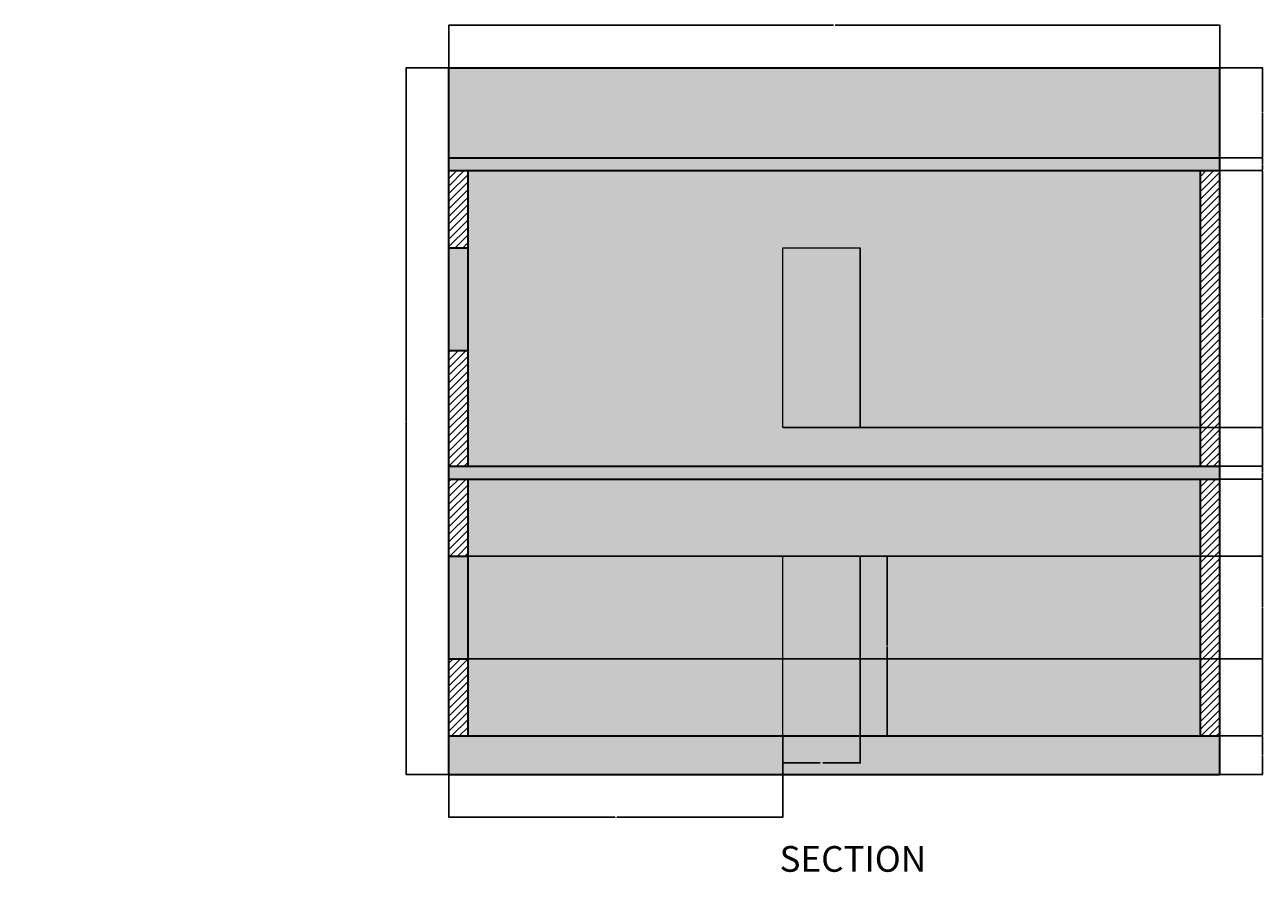
# Model space of a CAD drawing. Units: inches. Extents: x -43 to 1296, y -568 to 542.
# Tile 14 of 14: x 626 to 1204, y 83 to 479. Entities that reach past the tile are written whole.
import ezdxf

# ---------------------------------------------------------------- set-up
doc = ezdxf.new("R2010")
doc.units = ezdxf.units.IN
doc.header["$MEASUREMENT"] = 0
for name, color, linetype, lineweight in [('A-ANNO-DIMS', 2, 'Continuous', 18), ('A-ANNO-TEXT', 7, 'Continuous', 18), ('A-DOOR', 3, 'Continuous', 18), ('A-ELEV-OPEN-PATT', 13, 'Continuous', 13), ('A-SECT', 7, 'Continuous', 35), ('A-SECT-BASE-PATT', 222, 'Continuous', 13), ('A-WALL-PATT', 12, 'Continuous', 13)]:
    doc.layers.add(name, color=color, linetype=linetype, lineweight=lineweight)
for name, color, linetype, lineweight, true_color in [('A-ELEV-BAND-PATT', 30, 'Continuous', 13, 0xf8991e), ('A-ELEV-WALL-PATT', 31, 'Continuous', 13, 0xfecc66), ('A-ROOF-PATT', 217, 'Continuous', 13, 0x93278f)]:
    doc.layers.add(name, color=color, linetype=linetype, lineweight=lineweight, true_color=true_color)
doc.styles.get("Standard").update_dxf_attribs({"font": 'arial.ttf'})
doc.dimstyles.get("Standard").update_dxf_attribs({"dimtxt": 0.18, "dimasz": 0.18, "dimexe": 0.18, "dimexo": 0.0625, "dimgap": 0.09, "dimtad": 0, "dimtih": 1, "dimtoh": 1, "dimdec": 0, "dimzin": 0, "dimdsep": 46, "dimlunit": 3, "dimtxsty": 'Standard', "dimcen": 0.09, "dimadec": 0, "dimazin": 0, "dimtfac": 1, "dimtdec": 0, "dimtofl": 0, "dimtmove": 0, "dimatfit": 3, "dimfxl": 1, "dimtolj": 1, "dimtzin": 0, "dimarcsym": 0})

# ---------------------------------------------------------------- blocks, each defined once
blk = doc.blocks.new('DOOR-SECT-36x84')
for p, q in [((0, 0), (0, 84)), ((0, 84), (36, 84)), ((36, 0), (36, 84))]:
    blk.add_line(p, q)
blk = doc.blocks.new('*D56')
at = {"layer": 'A-ANNO-DIMS', "color": 0, "lineweight": -2, "transparency": 16777216}
for p, q in [((1016.19, 230.59), (1028.91, 230.59)), ((1028.73, 230.41), (1028.73, 188.77)), ((1028.73, 146.77), (1028.73, 188.41)), ((1016.19, 146.59), (1028.91, 146.59))]:
    blk.add_line(p, q, dxfattribs=at)
at = {"layer": 'A-ANNO-DIMS', "color": 0, "transparency": 16777216}
for points in [[(1028.7, 230.41), (1028.76, 230.41), (1028.73, 230.59)], [(1028.7, 146.77), (1028.76, 146.77), (1028.73, 146.59)]]:
    blk.add_solid(points, dxfattribs=at)
at = {"layer": 'Defpoints', "color": 0, "transparency": 16777216}
for p in [(1016.13, 230.59), (1028.73, 230.59), (1016.13, 146.59)]:
    blk.add_point(p, dxfattribs=at)
at = {"layer": 'A-ANNO-DIMS', "color": 0, "transparency": 16777216, "insert": (1028.73, 188.59), "char_height": 0.18, "attachment_point": 5}
blk.add_mtext('\\A1;DOOR 7\'-0" TYP.', dxfattribs=at)
blk = doc.blocks.new('*D57')
at = {"layer": 'A-ANNO-DIMS', "color": 0, "lineweight": -2, "transparency": 16777216}
for p, q in [((980.13, 146.53), (980.13, 133.81)), ((1016.13, 146.53), (1016.13, 133.81)), ((980.31, 133.99), (997.49, 133.99)), ((1015.95, 133.99), (998.77, 133.99))]:
    blk.add_line(p, q, dxfattribs=at)
at = {"layer": 'A-ANNO-DIMS', "color": 0, "transparency": 16777216}
for points in [[(980.31, 134.02), (980.31, 133.96), (980.13, 133.99)], [(1015.95, 134.02), (1015.95, 133.96), (1016.13, 133.99)]]:
    blk.add_solid(points, dxfattribs=at)
at = {"layer": 'Defpoints', "color": 0, "transparency": 16777216}
for p in [(980.13, 146.59), (1016.13, 146.59), (1016.13, 133.99)]:
    blk.add_point(p, dxfattribs=at)
at = {"layer": 'A-ANNO-DIMS', "color": 0, "transparency": 16777216, "insert": (998.13, 133.99), "char_height": 0.18, "attachment_point": 5}
blk.add_mtext('\\A1;3\'-0" TYP.', dxfattribs=at)
blk = doc.blocks.new('*D85')
at = {"layer": 'A-ANNO-DIMS', "color": 0, "lineweight": -2, "transparency": 16777216}
for p, q in [((824.13, 458.65), (824.13, 478.72)), ((824.31, 478.54), (1003.73, 478.54)), ((1183.95, 478.54), (1004.53, 478.54)), ((1184.13, 458.65), (1184.13, 478.72))]:
    blk.add_line(p, q, dxfattribs=at)
at = {"layer": 'A-ANNO-DIMS', "color": 0, "transparency": 16777216}
for points in [[(824.31, 478.57), (824.31, 478.51), (824.13, 478.54)], [(1183.95, 478.57), (1183.95, 478.51), (1184.13, 478.54)]]:
    blk.add_solid(points, dxfattribs=at)
at = {"layer": 'Defpoints', "color": 0, "transparency": 16777216}
for p in [(1184.13, 478.54), (824.13, 458.59), (1184.13, 458.59)]:
    blk.add_point(p, dxfattribs=at)
at = {"layer": 'A-ANNO-DIMS', "color": 0, "transparency": 16777216, "insert": (1004.13, 478.54), "char_height": 0.18, "attachment_point": 5}
blk.add_mtext('\\A1;30\'-0"', dxfattribs=at)
blk = doc.blocks.new('*D86')
at = {"layer": 'A-ANNO-DIMS', "color": 0, "lineweight": -2, "transparency": 16777216}
for p, q in [((824.07, 458.59), (804, 458.59)), ((804.18, 458.41), (804.18, 293.77)), ((804.18, 128.77), (804.18, 293.41)), ((824.07, 128.59), (804, 128.59))]:
    blk.add_line(p, q, dxfattribs=at)
at = {"layer": 'A-ANNO-DIMS', "color": 0, "transparency": 16777216}
for points in [[(804.15, 458.41), (804.21, 458.41), (804.18, 458.59)], [(804.15, 128.77), (804.21, 128.77), (804.18, 128.59)]]:
    blk.add_solid(points, dxfattribs=at)
at = {"layer": 'Defpoints', "color": 0, "transparency": 16777216}
for p in [(804.18, 458.59), (824.13, 458.59), (824.13, 128.59)]:
    blk.add_point(p, dxfattribs=at)
at = {"layer": 'A-ANNO-DIMS', "color": 0, "transparency": 16777216, "insert": (804.18, 293.59), "char_height": 0.18, "attachment_point": 5}
blk.add_mtext('\\A1;27\'-6"', dxfattribs=at)
blk = doc.blocks.new('*D87')
at = {"layer": 'A-ANNO-DIMS', "color": 0, "lineweight": -2, "transparency": 16777216}
for p, q in [((1184.19, 146.59), (1204.26, 146.59)), ((1204.08, 146.41), (1204.08, 137.77)), ((1204.08, 128.77), (1204.08, 137.41)), ((1184.19, 128.59), (1204.26, 128.59))]:
    blk.add_line(p, q, dxfattribs=at)
at = {"layer": 'A-ANNO-DIMS', "color": 0, "transparency": 16777216}
for points in [[(1204.05, 146.41), (1204.11, 146.41), (1204.08, 146.59)], [(1204.05, 128.77), (1204.11, 128.77), (1204.08, 128.59)]]:
    blk.add_solid(points, dxfattribs=at)
at = {"layer": 'Defpoints', "color": 0, "transparency": 16777216}
for p in [(1184.13, 146.59), (1204.08, 146.59), (1184.13, 128.59)]:
    blk.add_point(p, dxfattribs=at)
at = {"layer": 'A-ANNO-DIMS', "color": 0, "transparency": 16777216, "insert": (1204.08, 137.59), "char_height": 0.18, "attachment_point": 5}
blk.add_mtext('\\A1;1\'-6"', dxfattribs=at)
blk = doc.blocks.new('*D88')
at = {"layer": 'A-ANNO-DIMS', "color": 0, "lineweight": -2, "transparency": 16777216}
for p, q in [((1184.19, 266.59), (1204.26, 266.59)), ((1204.08, 266.41), (1204.08, 206.77)), ((1204.08, 146.77), (1204.08, 206.41)), ((1184.19, 146.59), (1204.26, 146.59))]:
    blk.add_line(p, q, dxfattribs=at)
at = {"layer": 'A-ANNO-DIMS', "color": 0, "transparency": 16777216}
for points in [[(1204.05, 266.41), (1204.11, 266.41), (1204.08, 266.59)], [(1204.05, 146.77), (1204.11, 146.77), (1204.08, 146.59)]]:
    blk.add_solid(points, dxfattribs=at)
at = {"layer": 'Defpoints', "color": 0, "transparency": 16777216}
for p in [(1184.13, 266.59), (1204.08, 266.59), (1184.13, 146.59)]:
    blk.add_point(p, dxfattribs=at)
at = {"layer": 'A-ANNO-DIMS', "color": 0, "transparency": 16777216, "insert": (1204.08, 206.59), "char_height": 0.18, "attachment_point": 5}
blk.add_mtext('\\A1;10\'-0"', dxfattribs=at)
blk = doc.blocks.new('*D89')
at = {"layer": 'A-ANNO-DIMS', "color": 0, "lineweight": -2, "transparency": 16777216}
for p, q in [((1184.19, 272.59), (1204.26, 272.59)), ((1204.08, 272.41), (1204.08, 269.77)), ((1184.19, 266.59), (1204.26, 266.59)), ((1204.08, 266.77), (1204.08, 269.41))]:
    blk.add_line(p, q, dxfattribs=at)
at = {"layer": 'A-ANNO-DIMS', "color": 0, "transparency": 16777216}
for points in [[(1204.05, 272.41), (1204.11, 272.41), (1204.08, 272.59)], [(1204.05, 266.77), (1204.11, 266.77), (1204.08, 266.59)]]:
    blk.add_solid(points, dxfattribs=at)
at = {"layer": 'Defpoints', "color": 0, "transparency": 16777216}
for p in [(1184.13, 272.59), (1204.08, 272.59), (1184.13, 266.59)]:
    blk.add_point(p, dxfattribs=at)
at = {"layer": 'A-ANNO-DIMS', "color": 0, "transparency": 16777216, "insert": (1204.08, 269.59), "char_height": 0.18, "attachment_point": 5}
blk.add_mtext('\\A1;0\'-6"', dxfattribs=at)
blk = doc.blocks.new('*D90')
at = {"layer": 'A-ANNO-DIMS', "color": 0, "lineweight": -2, "transparency": 16777216}
for p, q in [((1184.19, 410.59), (1204.26, 410.59)), ((1204.08, 410.41), (1204.08, 341.77)), ((1204.08, 272.77), (1204.08, 341.41)), ((1184.19, 272.59), (1204.26, 272.59))]:
    blk.add_line(p, q, dxfattribs=at)
at = {"layer": 'A-ANNO-DIMS', "color": 0, "transparency": 16777216}
for points in [[(1204.05, 410.41), (1204.11, 410.41), (1204.08, 410.59)], [(1204.05, 272.77), (1204.11, 272.77), (1204.08, 272.59)]]:
    blk.add_solid(points, dxfattribs=at)
at = {"layer": 'Defpoints', "color": 0, "transparency": 16777216}
for p in [(1184.13, 410.59), (1204.08, 410.59), (1184.13, 272.59)]:
    blk.add_point(p, dxfattribs=at)
at = {"layer": 'A-ANNO-DIMS', "color": 0, "transparency": 16777216, "insert": (1204.08, 341.59), "char_height": 0.18, "attachment_point": 5}
blk.add_mtext('\\A1;11\'-6"', dxfattribs=at)
blk = doc.blocks.new('*D91')
at = {"layer": 'A-ANNO-DIMS', "color": 0, "lineweight": -2, "transparency": 16777216}
for p, q in [((1184.19, 416.59), (1204.26, 416.59)), ((1204.08, 416.41), (1204.08, 413.77)), ((1204.08, 410.77), (1204.08, 413.41)), ((1184.19, 410.59), (1204.26, 410.59))]:
    blk.add_line(p, q, dxfattribs=at)
at = {"layer": 'A-ANNO-DIMS', "color": 0, "transparency": 16777216}
for points in [[(1204.05, 416.41), (1204.11, 416.41), (1204.08, 416.59)], [(1204.05, 410.77), (1204.11, 410.77), (1204.08, 410.59)]]:
    blk.add_solid(points, dxfattribs=at)
at = {"layer": 'Defpoints', "color": 0, "transparency": 16777216}
for p in [(1184.13, 416.59), (1204.08, 416.59), (1184.13, 410.59)]:
    blk.add_point(p, dxfattribs=at)
at = {"layer": 'A-ANNO-DIMS', "color": 0, "transparency": 16777216, "insert": (1204.08, 413.59), "char_height": 0.18, "attachment_point": 5}
blk.add_mtext('\\A1;0\'-6"', dxfattribs=at)
blk = doc.blocks.new('*D92')
at = {"layer": 'A-ANNO-DIMS', "color": 0, "lineweight": -2, "transparency": 16777216}
for p, q in [((1184.19, 458.59), (1204.26, 458.59)), ((1204.08, 458.41), (1204.08, 437.77)), ((1204.08, 416.77), (1204.08, 437.41)), ((1184.19, 416.59), (1204.26, 416.59))]:
    blk.add_line(p, q, dxfattribs=at)
at = {"layer": 'A-ANNO-DIMS', "color": 0, "transparency": 16777216}
for points in [[(1204.05, 458.41), (1204.11, 458.41), (1204.08, 458.59)], [(1204.05, 416.77), (1204.11, 416.77), (1204.08, 416.59)]]:
    blk.add_solid(points, dxfattribs=at)
at = {"layer": 'Defpoints', "color": 0, "transparency": 16777216}
for p in [(1184.13, 458.59), (1204.08, 458.59), (1184.13, 416.59)]:
    blk.add_point(p, dxfattribs=at)
at = {"layer": 'A-ANNO-DIMS', "color": 0, "transparency": 16777216, "insert": (1204.08, 437.59), "char_height": 0.18, "attachment_point": 5}
blk.add_mtext('\\A1;3\'-6"', dxfattribs=at)
blk = doc.blocks.new('*D93')
at = {"layer": 'A-ANNO-DIMS', "color": 0, "lineweight": -2, "transparency": 16777216}
for p, q in [((980.13, 146.53), (980.13, 108.46)), ((824.13, 128.53), (824.13, 108.46)), ((824.31, 108.64), (901.74, 108.64)), ((979.95, 108.64), (902.52, 108.64))]:
    blk.add_line(p, q, dxfattribs=at)
at = {"layer": 'A-ANNO-DIMS', "color": 0, "transparency": 16777216}
for points in [[(824.31, 108.67), (824.31, 108.61), (824.13, 108.64)], [(979.95, 108.67), (979.95, 108.61), (980.13, 108.64)]]:
    blk.add_solid(points, dxfattribs=at)
at = {"layer": 'Defpoints', "color": 0, "transparency": 16777216}
for p in [(980.13, 146.59), (824.13, 128.59), (980.13, 108.64)]:
    blk.add_point(p, dxfattribs=at)
at = {"layer": 'A-ANNO-DIMS', "color": 0, "transparency": 16777216, "insert": (902.13, 108.64), "char_height": 0.18, "attachment_point": 5}
blk.add_mtext('\\A1;13\'-0"', dxfattribs=at)
blk = doc.blocks.new('*D94')
at = {"layer": 'A-ANNO-DIMS', "color": 0, "lineweight": -2, "transparency": 16777216}
for p, q in [((833.19, 182.59), (1204.26, 182.59)), ((1204.08, 182.41), (1204.08, 164.77)), ((1204.08, 146.77), (1204.08, 164.41)), ((833.19, 146.59), (1204.26, 146.59))]:
    blk.add_line(p, q, dxfattribs=at)
at = {"layer": 'A-ANNO-DIMS', "color": 0, "transparency": 16777216}
for points in [[(1204.05, 182.41), (1204.11, 182.41), (1204.08, 182.59)], [(1204.05, 146.77), (1204.11, 146.77), (1204.08, 146.59)]]:
    blk.add_solid(points, dxfattribs=at)
at = {"layer": 'Defpoints', "color": 0, "transparency": 16777216}
for p in [(833.13, 182.59), (1204.08, 182.59), (833.13, 146.59)]:
    blk.add_point(p, dxfattribs=at)
at = {"layer": 'A-ANNO-DIMS', "color": 0, "transparency": 16777216, "insert": (1204.08, 164.59), "char_height": 0.18, "attachment_point": 5}
blk.add_mtext('\\A1;3\'-0"', dxfattribs=at)
blk = doc.blocks.new('*D95')
at = {"layer": 'A-ANNO-DIMS', "color": 0, "lineweight": -2, "transparency": 16777216}
for p, q in [((833.19, 230.59), (1204.26, 230.59)), ((1204.08, 230.41), (1204.08, 206.77)), ((1204.08, 182.77), (1204.08, 206.41)), ((833.19, 182.59), (1204.26, 182.59))]:
    blk.add_line(p, q, dxfattribs=at)
at = {"layer": 'A-ANNO-DIMS', "color": 0, "transparency": 16777216}
for points in [[(1204.05, 230.41), (1204.11, 230.41), (1204.08, 230.59)], [(1204.05, 182.77), (1204.11, 182.77), (1204.08, 182.59)]]:
    blk.add_solid(points, dxfattribs=at)
at = {"layer": 'Defpoints', "color": 0, "transparency": 16777216}
for p in [(833.13, 230.59), (1204.08, 230.59), (833.13, 182.59)]:
    blk.add_point(p, dxfattribs=at)
at = {"layer": 'A-ANNO-DIMS', "color": 0, "transparency": 16777216, "insert": (1204.08, 206.59), "char_height": 0.18, "attachment_point": 5}
blk.add_mtext('\\A1;4\'-0"', dxfattribs=at)
blk = doc.blocks.new('*D96')
at = {"layer": 'A-ANNO-DIMS', "color": 0, "lineweight": -2, "transparency": 16777216}
for p, q in [((980.19, 290.59), (1204.26, 290.59)), ((1204.08, 290.41), (1204.08, 281.77)), ((1204.08, 272.77), (1204.08, 281.41)), ((833.19, 272.59), (1204.26, 272.59))]:
    blk.add_line(p, q, dxfattribs=at)
at = {"layer": 'A-ANNO-DIMS', "color": 0, "transparency": 16777216}
for points in [[(1204.05, 290.41), (1204.11, 290.41), (1204.08, 290.59)], [(1204.05, 272.77), (1204.11, 272.77), (1204.08, 272.59)]]:
    blk.add_solid(points, dxfattribs=at)
at = {"layer": 'Defpoints', "color": 0, "transparency": 16777216}
for p in [(980.13, 290.59), (1204.08, 290.59), (833.13, 272.59)]:
    blk.add_point(p, dxfattribs=at)
at = {"layer": 'A-ANNO-DIMS', "color": 0, "transparency": 16777216, "insert": (1204.08, 281.59), "char_height": 0.18, "attachment_point": 5}
blk.add_mtext('\\A1;1\'-6"', dxfattribs=at)

msp = doc.modelspace()

# ---------------------------------------------------------------- hatches: boundary and pattern name
at = {"layer": 'A-ELEV-BAND-PATT'}
h = msp.add_hatch(color=256, dxfattribs=at)
h.dxf.hatch_style = 1
h.paths.add_polyline_path([(28.84, 332.29), (4.84, 332.29), (28.84, 320)])
h.paths.add_polyline_path([(412.84, 332.29), (388.84, 332.29), (388.84, 323.84)])
h.paths.add_polyline_path([(1184.13, 416.59), (824.13, 416.59), (824.13, 410.59), (1184.13, 410.59)])
h.paths.add_polyline_path([(1184.13, 272.59), (824.13, 272.59), (824.13, 266.59), (1184.13, 266.59)])
at = {"layer": 'A-ELEV-OPEN-PATT'}
h = msp.add_hatch(color=256, dxfattribs=at)
h.dxf.hatch_style = 1
h.paths.add_polyline_path([(79.84, 434.29), (43.84, 434.29), (43.84, 374.29), (79.84, 374.29)])
h.paths.add_polyline_path([(183.34, 434.29), (123.34, 434.29), (123.34, 386.29), (183.34, 386.29)])
h.paths.add_polyline_path([(337.84, 434.29), (277.84, 434.29), (277.84, 386.29), (337.84, 386.29)])
h.paths.add_polyline_path([(79.84, 290.29), (43.84, 290.29), (43.84, 248.29), (79.84, 248.29)])
h.paths.add_polyline_path([(183.34, 290.29), (123.34, 290.29), (123.34, 248.29), (183.34, 248.29)])
h.paths.add_polyline_path([(337.84, 290.29), (277.84, 290.29), (277.84, 248.29), (277.84, 230.87), (323.14, 248.29), (337.84, 242.64), (337.84, 248.29)])
h.paths.add_polyline_path([(1016.13, 374.59), (980.13, 374.59), (980.13, 290.59), (1016.13, 290.59)])
h.paths.add_polyline_path([(1016.13, 230.59), (980.13, 230.59), (980.13, 146.59), (1016.13, 146.59)])
h.paths.add_polyline_path([(833.13, 374.59), (824.13, 374.59), (824.13, 326.59), (833.13, 326.59)])
h.paths.add_polyline_path([(833.13, 230.59), (824.13, 230.59), (824.13, 182.59), (833.13, 182.59)])
at = {"layer": 'A-ELEV-WALL-PATT'}
h = msp.add_hatch(color=256, dxfattribs=at)
h.dxf.hatch_style = 1
h.paths.add_polyline_path([(1175.13, 410.59), (833.13, 410.59), (833.13, 272.59), (1175.13, 272.59)])
h.paths.add_polyline_path([(980.13, 374.59), (1016.13, 374.59), (1016.13, 290.59), (980.13, 290.59)], flags=16)
h = msp.add_hatch(color=256, dxfattribs=at)
h.dxf.hatch_style = 1
h.paths.add_polyline_path([(980.13, 230.59), (1016.13, 230.59), (1016.13, 146.59), (1175.13, 146.59), (1175.13, 266.59), (833.13, 266.59), (833.13, 146.59), (980.13, 146.59)])
at = {"layer": 'A-ROOF-PATT'}
h = msp.add_hatch(color=256, dxfattribs=at)
h.dxf.hatch_style = 1
h.paths.add_polyline_path([(1184.13, 458.59), (824.13, 458.59), (824.13, 416.59), (1184.13, 416.59)])
at = {"layer": 'A-SECT-BASE-PATT'}
h = msp.add_hatch(color=256, dxfattribs=at)
h.dxf.hatch_style = 1
h.paths.add_polyline_path([(1184.13, 146.59), (824.13, 146.59), (824.13, 128.59), (1184.13, 128.59)])
at = {"layer": 'A-WALL-PATT'}
h = msp.add_hatch(dxfattribs=at)
h.set_pattern_fill('ANSI31', color=256, scale=20)
h.paths.add_polyline_path([(833.13, 410.59), (824.13, 410.59), (824.13, 374.59), (833.13, 374.59)])
h.paths.add_polyline_path([(833.13, 326.59), (824.13, 326.59), (824.13, 272.59), (833.13, 272.59)])
h.paths.add_polyline_path([(833.13, 266.59), (824.13, 266.59), (824.13, 230.59), (833.13, 230.59)])
h.paths.add_polyline_path([(833.13, 182.59), (824.13, 182.59), (824.13, 146.59), (833.13, 146.59)])
h.paths.add_polyline_path([(1184.13, 266.59), (1175.13, 266.59), (1175.13, 146.59), (1184.13, 146.59)])
h.paths.add_polyline_path([(1184.13, 410.59), (1175.13, 410.59), (1175.13, 272.59), (1184.13, 272.59)])

# ---------------------------------------------------------------- linework, layer by layer
at = {"layer": 'A-DOOR'}
for points in [[(980.13, 374.59), (1016.13, 374.59), (1016.13, 290.59), (980.13, 290.59)], [(980.13, 230.59), (1016.13, 230.59), (1016.13, 146.59), (980.13, 146.59)]]:
    msp.add_lwpolyline(points, close=True, dxfattribs=at)
at = {"layer": 'A-SECT'}
for p, q in [((824.13, 272.59), (824.13, 458.59)), ((824.13, 458.59), (1184.13, 458.59)), ((1184.13, 272.59), (1184.13, 458.59)), ((824.13, 416.59), (1184.13, 416.59)), ((824.13, 410.59), (1184.13, 410.59)), ((833.13, 272.59), (833.13, 410.59)), ((1175.13, 272.59), (1175.13, 410.59)), ((824.13, 374.59), (833.13, 374.59)), ((824.13, 326.59), (833.13, 326.59)), ((824.13, 128.59), (824.13, 314.59)), ((1184.13, 128.59), (1184.13, 314.59)), ((824.13, 272.59), (1184.13, 272.59)), ((824.13, 266.59), (1184.13, 266.59)), ((833.13, 146.59), (833.13, 266.59)), ((1175.13, 146.59), (1175.13, 266.59)), ((824.13, 230.59), (833.13, 230.59)), ((824.13, 182.59), (833.13, 182.59)), ((824.13, 146.59), (1184.13, 146.59)), ((824.13, 128.59), (1184.13, 128.59))]:
    msp.add_line(p, q, dxfattribs=at)

# ---------------------------------------------------------------- block references
at = {"layer": 'A-DOOR'}
for p in [(980.13, 290.59), (980.13, 146.59)]:
    msp.add_blockref('DOOR-SECT-36x84', p, dxfattribs=at)

# ---------------------------------------------------------------- texts
at = {"layer": 'A-ANNO-TEXT', "insert": (978.57, 95.18), "char_height": 12, "attachment_point": 1}
msp.add_mtext('SECTION', dxfattribs=at)

# ---------------------------------------------------------------- dimensions: what is measured, and where the dimension line sits
at = {"layer": 'A-ANNO-DIMS'}
for base, p1, p2, picture, middle in [((1184.13, 478.54), (824.13, 458.59), (1184.13, 458.59), '*D85', (1004.13, 478.54)), ((980.13, 108.64), (824.13, 128.59), (980.13, 146.59), '*D93', (902.13, 108.64))]:
    dim = msp.add_linear_dim(base=base, p1=p1, p2=p2, dimstyle='Standard', override={"dimdec": 1, "dimlfac": 1, "dimrnd": 0, "dimzin": 1, "dimdsep": 46, "dimlunit": 4, "dimfrac": 2}, dxfattribs=at)
    dim.commit()
    dim.dimension.update_dxf_attribs({"geometry": picture, "text_midpoint": middle})
for base, p1, p2, picture, middle in [((804.18, 458.59), (824.13, 128.59), (824.13, 458.59), '*D86', (804.18, 293.59)), ((1204.08, 458.59), (1184.13, 416.59), (1184.13, 458.59), '*D92', (1204.08, 437.59)), ((1204.08, 416.59), (1184.13, 410.59), (1184.13, 416.59), '*D91', (1204.08, 413.59)), ((1204.08, 410.59), (1184.13, 272.59), (1184.13, 410.59), '*D90', (1204.08, 341.59)), ((1204.08, 290.59), (833.13, 272.59), (980.13, 290.59), '*D96', (1204.08, 281.59)), ((1204.08, 272.59), (1184.13, 266.59), (1184.13, 272.59), '*D89', (1204.08, 269.59)), ((1204.08, 266.59), (1184.13, 146.59), (1184.13, 266.59), '*D88', (1204.08, 206.59)), ((1204.08, 230.59), (833.13, 182.59), (833.13, 230.59), '*D95', (1204.08, 206.59)), ((1204.08, 182.59), (833.13, 146.59), (833.13, 182.59), '*D94', (1204.08, 164.59)), ((1204.08, 146.59), (1184.13, 128.59), (1184.13, 146.59), '*D87', (1204.08, 137.59))]:
    dim = msp.add_linear_dim(base=base, p1=p1, p2=p2, angle=90, dimstyle='Standard', override={"dimdec": 1, "dimlfac": 1, "dimrnd": 0, "dimzin": 1, "dimdsep": 46, "dimlunit": 4, "dimfrac": 2}, dxfattribs=at)
    dim.commit()
    dim.dimension.update_dxf_attribs({"geometry": picture, "text_midpoint": middle})
dim = msp.add_linear_dim(base=(1028.73, 230.59), p1=(1016.13, 146.59), p2=(1016.13, 230.59), angle=90, text='DOOR <> TYP.', dimstyle='Standard', override={"dimdec": 1, "dimlfac": 1, "dimrnd": 0, "dimzin": 1, "dimdsep": 46, "dimlunit": 4, "dimfrac": 2}, dxfattribs=at)
dim.commit()
dim.dimension.update_dxf_attribs({"geometry": '*D56', "text_midpoint": (1028.73, 188.59)})
dim = msp.add_linear_dim(base=(1016.13, 133.99), p1=(980.13, 146.59), p2=(1016.13, 146.59), text='<> TYP.', dimstyle='Standard', override={"dimdec": 1, "dimlfac": 1, "dimrnd": 0, "dimzin": 1, "dimdsep": 46, "dimlunit": 4, "dimfrac": 2}, dxfattribs=at)
dim.commit()
dim.dimension.update_dxf_attribs({"geometry": '*D57', "text_midpoint": (998.13, 133.99)})

doc.saveas('drawing.dxf')
